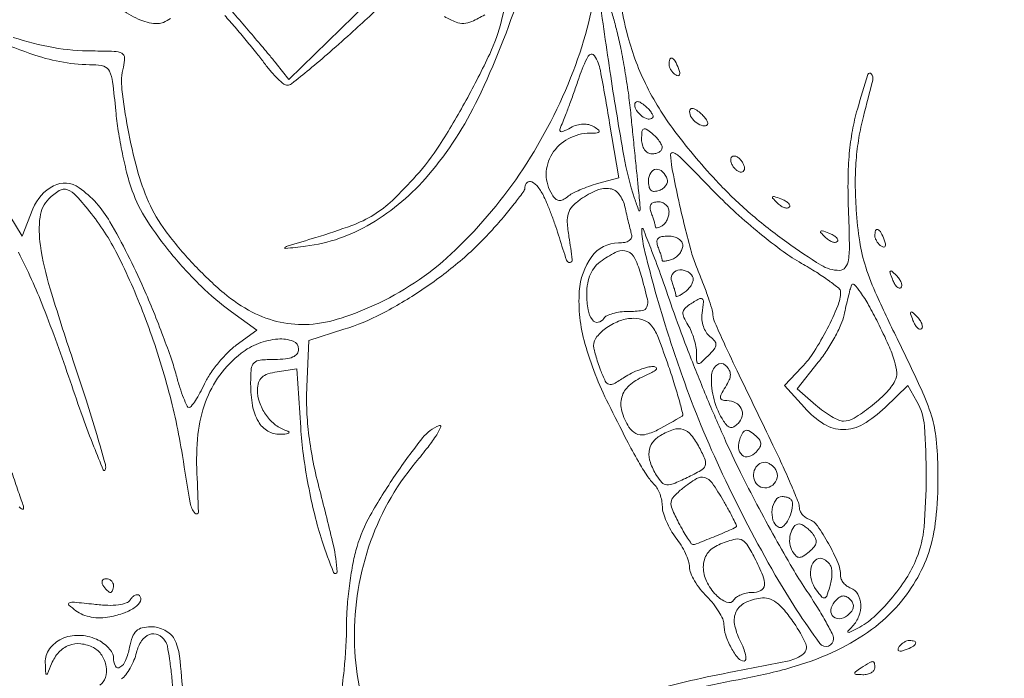
# Model space of a CAD drawing. Units: inches. Extents: x 2656 to 9931, y 1941 to 3068.
# Tile 36 of 46: x 2837 to 2847, y 2967 to 2974. Entities that reach past the tile are written whole.
import ezdxf

# ---------------------------------------------------------------- set-up
doc = ezdxf.new("R2010")
doc.units = ezdxf.units.IN
doc.layers.add('A-ANNO-DIMS', color=2, linetype='Continuous', lineweight=18)
doc.layers.add('A-ELEV-ORN', color=8, linetype='Continuous', lineweight=13)
doc.styles.get("Standard").update_dxf_attribs({"font": 'arial.ttf'})
doc.dimstyles.new('ISO-25', dxfattribs={"dimtxt": 6, "dimasz": 2.5, "dimexe": 1.25, "dimexo": 0.625, "dimtad": 1, "dimdec": 0, "dimlunit": 3, "dimtxsty": 'Standard', "dimcen": 2.5, "dimadec": 0, "dimazin": 0, "dimtfac": 1, "dimtdec": 0, "dimtmove": 0, "dimatfit": 3, "dimfxl": 1, "dimarcsym": 0})

# ---------------------------------------------------------------- blocks, each defined once
blk = doc.blocks.new('*D152')
at = {"layer": 'A-ANNO-DIMS', "color": 0, "lineweight": -2, "transparency": 16777216}
for p, q in [((2847.28, 2990.828), (2707.323, 2990.828)), ((2708.573, 2988.328), (2708.573, 2952.971)), ((2847.248, 2950.471), (2707.323, 2950.471))]:
    blk.add_line(p, q, dxfattribs=at)
at = {"layer": 'A-ANNO-DIMS', "color": 0, "transparency": 16777216}
for points in [[(2708.156, 2988.328), (2708.989, 2988.328), (2708.573, 2990.828)], [(2708.156, 2952.971), (2708.989, 2952.971), (2708.573, 2950.471)]]:
    blk.add_solid(points, dxfattribs=at)
at = {"layer": 'Defpoints', "color": 0, "transparency": 16777216}
for p in [(2847.905, 2990.828), (2708.573, 2950.471), (2847.873, 2950.471)]:
    blk.add_point(p, dxfattribs=at)
at = {"layer": 'A-ANNO-DIMS', "color": 0, "transparency": 16777216, "insert": (2704.843, 2970.649), "char_height": 6, "attachment_point": 5, "rotation": 90}
blk.add_mtext('3\'-4 1/2"', dxfattribs=at)
blk = doc.blocks.new('*D153')
at = {"layer": 'A-ANNO-DIMS', "color": 0, "lineweight": -2, "transparency": 16777216}
for p, q in [((2826.64, 2993.722), (2826.64, 2703.709)), ((2829.546, 2956.424), (2829.546, 2703.709)), ((2824.14, 2704.959), (2821.64, 2704.959)), ((2826.64, 2704.959), (2829.546, 2704.959)), ((2832.046, 2704.959), (2851.745, 2704.959))]:
    blk.add_line(p, q, dxfattribs=at)
at = {"layer": 'A-ANNO-DIMS', "color": 0, "transparency": 16777216}
for points in [[(2824.14, 2705.376), (2824.14, 2704.543), (2826.64, 2704.959)], [(2832.046, 2705.376), (2832.046, 2704.543), (2829.546, 2704.959)]]:
    blk.add_solid(points, dxfattribs=at)
at = {"layer": 'Defpoints', "color": 0, "transparency": 16777216}
for p in [(2826.64, 2994.347), (2829.546, 2957.049), (2829.546, 2704.959)]:
    blk.add_point(p, dxfattribs=at)
at = {"layer": 'A-ANNO-DIMS', "color": 0, "transparency": 16777216, "insert": (2843.145, 2708.65), "char_height": 6, "attachment_point": 5}
blk.add_mtext('0\'-3"', dxfattribs=at)
blk = doc.blocks.new('*D154')
at = {"layer": 'A-ANNO-DIMS', "color": 0, "lineweight": -2, "transparency": 16777216}
for p, q in [((2708.573, 2996.847), (2708.573, 2999.347)), ((2826.015, 2994.347), (2707.323, 2994.347)), ((2708.573, 2994.347), (2708.573, 2990.828)), ((2847.28, 2990.828), (2707.323, 2990.828)), ((2708.573, 2988.328), (2708.573, 2954.647))]:
    blk.add_line(p, q, dxfattribs=at)
at = {"layer": 'A-ANNO-DIMS', "color": 0, "transparency": 16777216}
for points in [[(2708.156, 2996.847), (2708.989, 2996.847), (2708.573, 2994.347)], [(2708.156, 2988.328), (2708.989, 2988.328), (2708.573, 2990.828)]]:
    blk.add_solid(points, dxfattribs=at)
at = {"layer": 'Defpoints', "color": 0, "transparency": 16777216}
for p in [(2826.64, 2994.347), (2708.573, 2990.828), (2847.905, 2990.828)]:
    blk.add_point(p, dxfattribs=at)
at = {"layer": 'A-ANNO-DIMS', "color": 0, "transparency": 16777216, "insert": (2704.843, 2970.237), "char_height": 6, "attachment_point": 5, "rotation": 90}
blk.add_mtext('0\'-3 1/2"', dxfattribs=at)

msp = doc.modelspace()

# ---------------------------------------------------------------- linework, layer by layer
at = {"layer": 'A-ELEV-ORN'}
for points in [[(2842.853, 2974.397, -0.062714), (2842.597, 2973.361, -0.053881), (2842.084, 2972.363, -0.0556), (2841.391, 2971.531, -0.080212), (2840.605, 2970.986, -0.032224), (2840.218, 2970.831, -0.061455), (2839.891, 2970.767, -0.072265), (2839.594, 2970.789, -0.065114), (2839.305, 2970.893, -0.056633), (2839.017, 2971.087, -0.028415), (2838.699, 2971.389, -0.028415), (2838.418, 2971.725, -0.056908), (2838.244, 2972.024, -0.036526), (2838.126, 2972.358, -0.020375), (2838.03, 2972.778, -0.018439), (2837.97, 2973.178, -0.089515), (2837.985, 2973.406, 0.061039), (2837.997, 2973.502, 0.280443), (2837.969, 2973.548, 0.112433), (2837.892, 2973.568, 0.00783), (2837.667, 2973.572, -0.044024), (2837.268, 2973.607, -0.036465), (2836.854, 2973.712, -0.031934)], [(2843.31, 2966.892, -0.021083), (2844.354, 2967.133, 0.026141), (2844.873, 2967.258, 0.039837), (2845.306, 2967.425, 0.045741), (2845.658, 2967.636, 0.058065), (2845.936, 2967.893, 0.04841), (2846.13, 2968.171, 0.05757), (2846.255, 2968.465, 0.049384), (2846.321, 2968.816, 0.024614), (2846.338, 2969.268, 0.021923), (2846.32, 2969.588, 0.049336), (2846.272, 2969.827, 0.034106), (2846.168, 2970.099, 0.006116), (2845.934, 2970.591, -0.007097), (2845.711, 2971.062, -0.029397), (2845.597, 2971.355, -0.039713), (2845.536, 2971.615, -0.021446), (2845.5, 2971.941, -0.015651), (2845.49, 2972.208, -0.020354), (2845.499, 2972.452, -0.021729), (2845.527, 2972.681, -0.023377), (2845.574, 2972.901, 0.004012), (2845.669, 2973.272, 0.238331), (2845.654, 2973.338, 0.595051), (2845.619, 2973.331, 0.00437), (2845.512, 2972.975, 0.026292), (2845.461, 2972.757, 0.0221), (2845.429, 2972.521, 0.019508), (2845.416, 2972.256, 0.012547), (2845.42, 2971.948, -0.005025), (2845.43, 2971.592, -0.041002), (2845.42, 2971.43, -0.122762), (2845.388, 2971.351, -0.238712), (2845.328, 2971.321, -0.138821), (2845.139, 2971.375, -0.018176), (2844.788, 2971.609, -0.021642), (2844.414, 2971.904, -0.026108), (2844.091, 2972.213, -0.027001), (2843.64, 2972.747, -0.048186), (2843.339, 2973.237, -0.051403), (2843.15, 2973.753, -0.035809), (2843.041, 2974.363, 0.011612)], [(2839.024, 2973.936, -0.00618), (2839.13, 2973.816, -0.004408), (2839.245, 2973.68, -0.004451), (2839.353, 2973.547, -0.00948), (2839.433, 2973.443, 0.018291), (2839.501, 2973.358, 0.024307), (2839.569, 2973.286, 0.022933), (2839.63, 2973.233, 0.169618), (2839.666, 2973.22, 0.170059), (2839.71, 2973.236, 0.003586), (2839.892, 2973.383, 0.007897), (2840.104, 2973.563, 0.005188), (2840.342, 2973.776, -0.00338), (2840.721, 2974.118, -0.04635)], [(2841.908, 2974.067), (2841.863, 2973.884, -0.047953), (2841.741, 2973.541, -0.016187), (2841.5, 2973.067, -0.016433), (2841.226, 2972.605, -0.041092), (2840.988, 2972.293, -0.017871), (2840.743, 2972.039, -0.053766), (2840.552, 2971.891, -0.050229), (2840.328, 2971.782, -0.014129), (2839.958, 2971.658, 0.000751), (2839.673, 2971.571, 0.101126), (2839.641, 2971.554, 0.742785), (2839.645, 2971.545, 0.00203), (2839.853, 2971.569, 0.104505), (2840.525, 2971.801, 0.082382), (2841.114, 2972.3, 0.064174), (2841.622, 2973.085, 0.033435), (2842.054, 2974.17, 0.022106)], [(2840.483, 2974.058), (2839.681, 2973.279), (2839.552, 2973.443, 0.007333), (2839.48, 2973.532, 0.001692), (2839.355, 2973.68, 0.001747), (2839.211, 2973.849, 0.001706), (2839.065, 2974.018)], [(2837.973, 2973.995, 0.057004), (2838.163, 2973.889, 0.09937), (2838.34, 2973.853, 0.108281), (2838.395, 2973.865, 0.034437), (2838.468, 2973.905, 0.032541)], [(2841.278, 2973.925, 0.028926), (2841.396, 2973.869, 0.107992), (2841.476, 2973.855, 0.097967), (2841.559, 2973.875, 0.02151), (2841.69, 2973.942)], [(2836.272, 2973.858, 0.029582), (2837.076, 2973.53, 0.082237), (2837.675, 2973.431, -0.074513), (2837.785, 2973.415, -0.207271), (2837.843, 2973.365, -0.084093), (2837.875, 2973.256, -0.006773), (2837.907, 2972.957, 0.015972), (2837.933, 2972.751, 0.011369), (2837.975, 2972.521, 0.011495), (2838.025, 2972.303, 0.023883), (2838.076, 2972.137, 0.057669), (2838.224, 2971.837, 0.028184), (2838.475, 2971.493, 0.027587), (2838.78, 2971.161, 0.036635), (2839.093, 2970.897), (2839.353, 2970.709), (2839.142, 2970.553, 0.038605), (2839.053, 2970.476, 0.023263), (2838.96, 2970.372, 0.023225), (2838.876, 2970.26, 0.037249), (2838.817, 2970.156, -0.013462), (2838.769, 2970.063, -0.020038), (2838.723, 2969.985, -0.015751), (2838.681, 2969.925, -0.236477), (2838.659, 2969.914, -0.294197), (2838.638, 2969.928, -0.012177), (2838.602, 2970.012, -0.017773), (2838.564, 2970.118, -0.011292), (2838.527, 2970.245, 0.018154), (2838.477, 2970.41, 0.00638), (2838.393, 2970.644, 0.006324), (2838.293, 2970.898, 0.007367), (2838.192, 2971.137, 0.027175), (2837.847, 2971.82, 0.106386), (2837.531, 2972.169, 0.282935), (2837.269, 2972.188, 0.181331), (2837.058, 2971.953), (2836.947, 2971.671), (2836.821, 2971.88, 0.042011)], [(2836.908, 2971.506, -0.025971), (2837.163, 2970.944, -0.011782), (2837.439, 2970.186, 0.004309), (2837.569, 2969.813, 0.007894), (2837.683, 2969.511, 0.00415), (2837.779, 2969.273, 0.694448), (2837.799, 2969.274, 0.150521), (2837.8, 2969.33, 0.00245), (2837.712, 2969.637, 0.006144), (2837.602, 2969.994, 0.00401), (2837.467, 2970.404, -0.008425), (2837.234, 2971.133, -0.036079), (2837.134, 2971.577, -0.066195), (2837.13, 2971.868, -0.168907), (2837.22, 2972.055, -0.059645), (2837.328, 2972.139, -0.224773), (2837.411, 2972.148, -0.127121), (2837.501, 2972.087, -0.015227), (2837.657, 2971.901, -0.052466), (2837.939, 2971.454, -0.024343), (2838.213, 2970.822, -0.023509), (2838.441, 2970.114, -0.027309), (2838.59, 2969.422, 0.003756), (2838.671, 2968.934, 0.128056), (2838.719, 2968.828, 0.715598), (2838.754, 2968.84, 0.006631), (2838.739, 2969.238, -0.038668), (2838.75, 2969.638, -0.062097), (2838.827, 2969.971, -0.070148), (2838.974, 2970.245, -0.068088), (2839.192, 2970.47, -0.075108), (2839.37, 2970.571, -0.074118), (2839.57, 2970.616, -0.104512), (2839.725, 2970.595, -0.316192), (2839.782, 2970.512, -0.164293), (2839.767, 2970.465, -0.129352), (2839.724, 2970.432, -0.075863), (2839.649, 2970.413, -0.025511), (2839.536, 2970.407, 0.021968), (2839.386, 2970.4, 0.178574), (2839.325, 2970.371, 0.174885), (2839.296, 2970.309, 0.020892), (2839.29, 2970.156, 0.043336), (2839.309, 2969.933, 0.088805), (2839.369, 2969.77, 0.125073), (2839.466, 2969.671, 0.14633), (2839.591, 2969.639, 0.01274), (2839.658, 2969.643, 0.157257), (2839.681, 2969.652, 0.524361), (2839.679, 2969.665, 0.039035), (2839.642, 2969.682, -0.088287), (2839.533, 2969.744, -0.069673), (2839.442, 2969.844, -0.068701), (2839.381, 2969.967, -0.080851), (2839.36, 2970.096, -0.073644), (2839.372, 2970.171, -0.135274), (2839.404, 2970.223, -0.109805), (2839.465, 2970.258, -0.038951), (2839.562, 2970.28), (2839.764, 2970.309), (2839.803, 2969.707, 0.017712), (2839.831, 2969.426, 0.013084), (2839.881, 2969.116, 0.013118), (2839.947, 2968.811, 0.018296), (2840.023, 2968.543, 0.018649), (2840.141, 2968.221, 0.84301), (2840.176, 2968.229, 0.046019), (2840.138, 2968.499, 0.006058), (2839.999, 2969.062, -0.014444), (2839.932, 2969.352, -0.018534), (2839.888, 2969.623, -0.019852), (2839.866, 2969.879, -0.022359), (2839.866, 2970.126), (2839.888, 2970.602), (2840.247, 2970.716, 0.042983), (2840.632, 2970.875, 0.028302), (2841.045, 2971.12, 0.027738), (2841.439, 2971.417, 0.034228), (2841.769, 2971.738, 0.007807), (2841.897, 2971.885, 0.011327), (2842.005, 2972.019, 0.007101), (2842.091, 2972.134, 0.158019), (2842.103, 2972.173, -0.212493), (2842.126, 2972.222, -0.306704), (2842.172, 2972.229, -0.116091), (2842.237, 2972.175, -0.049272), (2842.298, 2972.077, -0.017168), (2842.333, 2971.998, -0.006886), (2842.376, 2971.888, -0.006804), (2842.419, 2971.768, -0.008541), (2842.456, 2971.655, 0.006236), (2842.529, 2971.425, 0.346324), (2842.565, 2971.402, 0.428109), (2842.588, 2971.43, 0.006685), (2842.554, 2971.664, -0.02305), (2842.537, 2971.815, -0.092243), (2842.548, 2971.907, -0.116837), (2842.589, 2971.978, -0.048286), (2842.674, 2972.05, -0.051712), (2842.842, 2972.144, -0.145026), (2842.975, 2972.159, -0.194836), (2843.07, 2972.1, -0.103782), (2843.128, 2971.972, 0.003398), (2843.146, 2971.891, 0.003194), (2843.166, 2971.809, 0.003177), (2843.184, 2971.737, 0.011017), (2843.197, 2971.69, -0.172957), (2843.196, 2971.655, -0.153568), (2843.172, 2971.627, -0.098751), (2843.126, 2971.608, -0.045369), (2843.062, 2971.602, 0.240793), (2842.787, 2971.462, 0.141871), (2842.66, 2971.107, 0.085228), (2842.718, 2970.57, 0.046137), (2842.959, 2969.95, 0.002777), (2843.145, 2969.581, 0.011089), (2843.266, 2969.359, 0.01768), (2843.356, 2969.213, 0.049192), (2843.432, 2969.121, -0.072159), (2843.462, 2969.08, -0.03806), (2843.488, 2969.023, -0.0369), (2843.505, 2968.959, -0.046713), (2843.512, 2968.898, 0.069701), (2843.522, 2968.83, 0.030218), (2843.553, 2968.745, 0.029173), (2843.598, 2968.656, 0.03429), (2843.651, 2968.578, -0.03034), (2843.704, 2968.501, -0.027752), (2843.748, 2968.417, -0.028834), (2843.78, 2968.337, -0.076098), (2843.79, 2968.276, 0.096524), (2843.803, 2968.215, 0.033427), (2843.843, 2968.135, 0.031738), (2843.9, 2968.05, 0.031897), (2843.967, 2967.974, -0.027616), (2844.035, 2967.899, -0.029667), (2844.092, 2967.818, -0.03103), (2844.132, 2967.744, -0.108485), (2844.143, 2967.691, 0.080423), (2844.162, 2967.577, 0.045303), (2844.218, 2967.448, 0.044022), (2844.289, 2967.342, 0.226965), (2844.351, 2967.312, 0.397473), (2844.368, 2967.327, 0.065356), (2844.364, 2967.375, 0.04263), (2844.344, 2967.444, 0.022195), (2844.307, 2967.526, -0.070131), (2844.252, 2967.691, -0.159908), (2844.269, 2967.82, -0.166772), (2844.359, 2967.91, -0.077793), (2844.518, 2967.959, -0.108309), (2844.6, 2967.954, -0.089808), (2844.679, 2967.914, -0.06072), (2844.763, 2967.834, -0.021767), (2844.862, 2967.702, -0.042697), (2844.983, 2967.488, -0.342151), (2844.958, 2967.385, -0.119272), (2844.812, 2967.316, -0.005091), (2844.248, 2967.204, 0.020325), (2843.366, 2967.002, 0.031031)], [(2840.565, 2966.551, -0.095957), (2840.355, 2967.471, -0.087707), (2840.5, 2968.48, -0.09438), (2840.982, 2969.35, 0.009507), (2841.109, 2969.508, 0.021327), (2841.198, 2969.635, 0.038848), (2841.241, 2969.714, 0.666896), (2841.226, 2969.729, 0.135525), (2841.052, 2969.601, 0.01693), (2840.773, 2969.22, 0.020826), (2840.516, 2968.806, 0.056534), (2840.381, 2968.489, 0.024973), (2840.34, 2968.321, 0.013411), (2840.306, 2968.111, 0.013323), (2840.282, 2967.893, 0.020314), (2840.274, 2967.704, -0.026531), (2840.248, 2967.219, -0.015759), (2840.169, 2966.645, -0.015384)], [(2836.916, 2968.895, 0.046443), (2836.947, 2968.87, 0.495533), (2836.959, 2968.875, 0.152674), (2836.959, 2968.901, 0.013093), (2836.938, 2968.965, -0.007722), (2836.907, 2969.052, -0.000935), (2836.843, 2969.243, -0.001111)], [(2838.598, 2966.947, 0.010925), (2838.56, 2967.362, 0.092946), (2838.506, 2967.541, 0.095655), (2838.468, 2967.588, 0.058053), (2838.409, 2967.628, 0.05525), (2838.338, 2967.655, 0.063506), (2838.266, 2967.664, 0.059093), (2838.177, 2967.653, 0.13444), (2838.118, 2967.621, 0.114543), (2838.078, 2967.559, 0.036658), (2838.049, 2967.453, -0.046905), (2838.008, 2967.318, -0.157361), (2837.95, 2967.248, -0.448318), (2837.903, 2967.261, -0.11211), (2837.883, 2967.349, 0.1326), (2837.871, 2967.395, 0.056806), (2837.832, 2967.448, 0.050694), (2837.775, 2967.497, 0.046624), (2837.708, 2967.536, 0.103136), (2837.528, 2967.576, 0.112073), (2837.353, 2967.54, 0.129566), (2837.228, 2967.437, 0.164796), (2837.184, 2967.296, 0.0025), (2837.188, 2967.185, 0.353585), (2837.196, 2967.176, 0.351009), (2837.207, 2967.182, 0.002485), (2837.249, 2967.285, -0.088994), (2837.323, 2967.402, -0.116417), (2837.427, 2967.473, -0.119244), (2837.55, 2967.489, -0.096506), (2837.677, 2967.45, -0.125381), (2837.763, 2967.372, -0.103427), (2837.808, 2967.256, -0.114975), (2837.801, 2967.142, -0.183925), (2837.743, 2967.066, 0.107671)], [(2837.964, 2967.128, 0.071928), (2838.009, 2967.171, 0.032471), (2838.054, 2967.24, 0.031305), (2838.093, 2967.32, 0.037148), (2838.119, 2967.4, -0.084654), (2838.171, 2967.519, -0.155138), (2838.253, 2967.585, -0.204368), (2838.341, 2967.582, -0.14709), (2838.415, 2967.516, -0.091318), (2838.436, 2967.464, -0.009542), (2838.458, 2967.334, -0.01158), (2838.478, 2967.178, -0.009031), (2838.493, 2967.006, 0.010541)]]:
    msp.add_lwpolyline(points, format="xyb", dxfattribs=at)
for points in [[(2843.046, 2973.776, -0.013205), (2843.086, 2973.598, -0.006854), (2843.127, 2973.373, -0.00681), (2843.163, 2973.142, -0.010294), (2843.187, 2972.939, 0.000202), (2843.207, 2972.741, 0.000153), (2843.229, 2972.523, 0.000154), (2843.25, 2972.318, 0.000358), (2843.265, 2972.165, -0.001534), (2843.285, 2971.967, -0.110402), (2843.281, 2971.935, -0.7056), (2843.27, 2971.935, -0.004671), (2843.227, 2972.06, -0.036376), (2843.117, 2972.496, -0.006701), (2842.982, 2973.315, -0.002798), (2842.858, 2974.173, -0.711672), (2842.906, 2974.198, -0.114458), (2842.927, 2974.165, -0.007415), (2842.965, 2974.057, -0.010497), (2843.006, 2973.924, -0.007618)], [(2842.971, 2972.833), (2843.064, 2972.271), (2842.848, 2972.212, 0.01944), (2842.758, 2972.183, 0.017473), (2842.667, 2972.147, 0.017805), (2842.588, 2972.109, 0.051355), (2842.538, 2972.075, -0.055462), (2842.49, 2972.044, -0.15622), (2842.451, 2972.038, -0.158077), (2842.416, 2972.055, -0.057176), (2842.381, 2972.099, -0.143378), (2842.321, 2972.306, -0.137922), (2842.381, 2972.516, -0.130656), (2842.546, 2972.671, -0.123085), (2842.77, 2972.729, 0.012592), (2842.844, 2972.731, 0.243204), (2842.863, 2972.743, 0.387784), (2842.86, 2972.76, 0.021395), (2842.811, 2972.794, 0.083301), (2842.759, 2972.816, 0.067688), (2842.699, 2972.822, 0.062021), (2842.635, 2972.811, 0.051282), (2842.571, 2972.785, -0.012015), (2842.492, 2972.745, -0.272927), (2842.468, 2972.747, -0.336052), (2842.461, 2972.768, -0.015615), (2842.491, 2972.843, 0.012129), (2842.52, 2972.914, 0.003033), (2842.564, 2973.033, 0.003097), (2842.613, 2973.169, 0.003111), (2842.66, 2973.305, -0.037921), (2842.751, 2973.519, -0.573274), (2842.816, 2973.522, -0.100097), (2842.876, 2973.372, -0.00472)], [(2843.58, 2973.435, 0.088797), (2843.586, 2973.407, 0.053277), (2843.601, 2973.376, 0.051183), (2843.623, 2973.347, 0.061454), (2843.65, 2973.326, 0.1144), (2843.674, 2973.318, 0.32948), (2843.688, 2973.327, 0.155351), (2843.69, 2973.352, 0.036408), (2843.678, 2973.392, 0.029964), (2843.643, 2973.468, 0.168622), (2843.612, 2973.497, 0.444011), (2843.589, 2973.487, 0.079093)], [(2843.411, 2972.887, -0.264952), (2843.365, 2972.874, -0.097357), (2843.302, 2972.904, -0.084765), (2843.248, 2972.961, -0.149534), (2843.229, 2973.022, -0.176123), (2843.237, 2973.045, -0.256649), (2843.257, 2973.053, -0.110288), (2843.291, 2973.041, -0.030483), (2843.336, 2973.008, -0.030935), (2843.375, 2972.971, -0.05004), (2843.402, 2972.935, -0.066988), (2843.416, 2972.905, -0.274667)], [(2843.791, 2972.952, 0.149534), (2843.81, 2972.89, 0.084765), (2843.864, 2972.834, 0.097357), (2843.928, 2972.804, 0.264952), (2843.974, 2972.816, 0.274667), (2843.978, 2972.835, 0.066988), (2843.965, 2972.865, 0.05004), (2843.937, 2972.901, 0.030935), (2843.899, 2972.937, 0.030483), (2843.853, 2972.971, 0.110288), (2843.82, 2972.983, 0.256649), (2843.8, 2972.975, 0.176123)], [(2843.51, 2972.579, -0.167044), (2843.502, 2972.555, -0.095133), (2843.479, 2972.535, -0.075975), (2843.445, 2972.521, -0.056567), (2843.405, 2972.517, -0.132926), (2843.363, 2972.528, -0.107148), (2843.329, 2972.559, -0.089651), (2843.307, 2972.607, -0.064485), (2843.299, 2972.666, -0.02153), (2843.303, 2972.745, -0.243483), (2843.319, 2972.771, -0.285199), (2843.347, 2972.77, -0.027702), (2843.405, 2972.728, -0.031583), (2843.445, 2972.69, -0.034151), (2843.479, 2972.648, -0.036411), (2843.503, 2972.608, -0.117955)], [(2844.939, 2971.393, -0.011671), (2845.092, 2971.301, -0.017384), (2845.221, 2971.214, -0.012556), (2845.322, 2971.137, -0.226393), (2845.339, 2971.101, -0.097548), (2845.31, 2970.956, -0.021009), (2845.203, 2970.722, -0.022913), (2845.069, 2970.489, -0.049851), (2844.942, 2970.326), (2844.764, 2970.141), (2844.968, 2969.913, 0.070733), (2845.168, 2969.744, 0.140656), (2845.366, 2969.688, 0.133051), (2845.571, 2969.743, 0.060285), (2845.795, 2969.913), (2846.029, 2970.14), (2846.123, 2969.975, -0.112118), (2846.2, 2969.722, -0.018342), (2846.217, 2969.207, -0.020283), (2846.195, 2968.686, -0.074855), (2846.119, 2968.367, -0.046499), (2846.012, 2968.159, -0.032722), (2845.855, 2967.947, -0.033275), (2845.68, 2967.764, -0.065122), (2845.515, 2967.649, -0.004388), (2845.435, 2967.609, -0.209201), (2845.418, 2967.608, -0.523579), (2845.415, 2967.618, -0.008587), (2845.462, 2967.669, 0.099511), (2845.527, 2967.773, 0.10171), (2845.546, 2967.894, 0.118463), (2845.516, 2967.998, 0.173667), (2845.444, 2968.06, -0.066404), (2845.404, 2968.082, -0.062204), (2845.37, 2968.114, -0.066541), (2845.347, 2968.152, -0.106625), (2845.339, 2968.188, 0.100816), (2845.312, 2968.322, 0.027214), (2845.216, 2968.517, 0.02503), (2845.102, 2968.699, 0.149487), (2845.015, 2968.767, -0.066359), (2844.977, 2968.787, -0.062579), (2844.946, 2968.817, -0.067076), (2844.924, 2968.851, -0.107584), (2844.917, 2968.884, 0.097311), (2844.907, 2968.938, 0.004626), (2844.838, 2969.107, 0.007446), (2844.75, 2969.306, 0.005277), (2844.646, 2969.528, -0.000529), (2844.299, 2970.247, -0.004156), (2844.141, 2970.583, -0.005965), (2844.051, 2970.785, -0.077965), (2844.031, 2970.864, 0.046602), (2844.018, 2970.931, 0.01196), (2843.984, 2971.037, 0.009849), (2843.934, 2971.176, 0.004445), (2843.862, 2971.356, -0.029497), (2843.81, 2971.508, -0.00682), (2843.742, 2971.768, -0.007038), (2843.672, 2972.071, -0.006934), (2843.61, 2972.376, -0.04477), (2843.597, 2972.508, -0.580404), (2843.631, 2972.528, -0.06677), (2843.719, 2972.459, -0.001932), (2844.051, 2972.12, 0.015764), (2844.267, 2971.912, 0.012488), (2844.513, 2971.699, 0.012678), (2844.752, 2971.514, 0.030532)], [(2844.213, 2972.455, 0.085235), (2844.219, 2972.425, 0.053414), (2844.234, 2972.392, 0.051777), (2844.257, 2972.363, 0.064269), (2844.284, 2972.341, 0.076764), (2844.311, 2972.33, 0.154201), (2844.333, 2972.331, 0.186277), (2844.349, 2972.344, 0.117858), (2844.354, 2972.368, 0.085235), (2844.349, 2972.398, 0.053414), (2844.333, 2972.43, 0.051777), (2844.311, 2972.46, 0.064269), (2844.284, 2972.482, 0.076764), (2844.257, 2972.493, 0.154201), (2844.234, 2972.492, 0.186277), (2844.219, 2972.478, 0.117858)], [(2843.561, 2972.257, -0.142819), (2843.563, 2972.226, -0.094374), (2843.547, 2972.192, -0.080169), (2843.518, 2972.162, -0.065676), (2843.478, 2972.141, -0.081514), (2843.429, 2972.131, -0.202481), (2843.395, 2972.143, -0.158084), (2843.375, 2972.18, -0.046434), (2843.369, 2972.244, -0.135971), (2843.392, 2972.323, -0.244334), (2843.448, 2972.358, -0.216449), (2843.514, 2972.333, -0.117556)], [(2843.58, 2971.923, -0.061875), (2843.575, 2971.881, -0.051278), (2843.56, 2971.839, -0.053305), (2843.537, 2971.802, -0.08825), (2843.51, 2971.778, -0.033138), (2843.483, 2971.764, -0.070413), (2843.46, 2971.757, -0.136025), (2843.446, 2971.759, -0.30111), (2843.44, 2971.768, 0.061959), (2843.437, 2971.788, 0.00979), (2843.427, 2971.825, 0.010735), (2843.413, 2971.868, 0.009199), (2843.397, 2971.913, -0.067159), (2843.386, 2971.961, -0.16701), (2843.394, 2971.996, -0.176865), (2843.421, 2972.017, -0.076855), (2843.467, 2972.024, -0.088448), (2843.511, 2972.017, -0.094811), (2843.547, 2971.995, -0.099989), (2843.572, 2971.962, -0.110744)], [(2844.687, 2972.016, 0.043285), (2844.723, 2971.985, 0.063152), (2844.76, 2971.966, 0.082976), (2844.792, 2971.959, 0.20742), (2844.813, 2971.968, 0.278911), (2844.818, 2971.987, 0.120343), (2844.804, 2972.01, 0.070189), (2844.772, 2972.034, 0.036269), (2844.726, 2972.055, 0.008399), (2844.659, 2972.079, 0.286372), (2844.643, 2972.076, 0.400052), (2844.643, 2972.062, 0.011214)], [(2844.314, 2969.246, 0.006536), (2844.482, 2968.919, 0.005449), (2844.668, 2968.576, 0.005504), (2844.846, 2968.265, 0.014889), (2844.981, 2968.051, -0.008625), (2845.09, 2967.882, -0.011652), (2845.182, 2967.727, -0.008777), (2845.253, 2967.594, -0.113511), (2845.267, 2967.541, -0.733514), (2845.127, 2967.493, -0.027589), (2844.67, 2968.194, -0.020379), (2844.13, 2969.229, -0.025468), (2843.718, 2970.231, -0.007961), (2843.558, 2970.707, -0.009529), (2843.424, 2971.161, -0.008632), (2843.325, 2971.546, -0.056718), (2843.301, 2971.743, -0.824628), (2843.314, 2971.746, -0.005289), (2843.392, 2971.549, -0.00641), (2843.494, 2971.278, -0.003255), (2843.614, 2970.934, 0.009355), (2843.763, 2970.528, 0.005983), (2843.949, 2970.061, 0.006011), (2844.144, 2969.608, 0.011157)], [(2845.179, 2971.664, 0.043285), (2845.216, 2971.633, 0.063152), (2845.252, 2971.614, 0.082976), (2845.284, 2971.608, 0.20742), (2845.306, 2971.616, 0.278911), (2845.31, 2971.635, 0.120343), (2845.296, 2971.658, 0.070189), (2845.264, 2971.682, 0.036269), (2845.219, 2971.703, 0.008399), (2845.151, 2971.728, 0.286372), (2845.136, 2971.724, 0.400052), (2845.135, 2971.71, 0.011214)], [(2845.691, 2971.677, 0.088797), (2845.696, 2971.648, 0.053277), (2845.711, 2971.618, 0.051183), (2845.733, 2971.589, 0.061454), (2845.76, 2971.568, 0.1144), (2845.784, 2971.56, 0.32948), (2845.798, 2971.568, 0.155351), (2845.8, 2971.593, 0.036408), (2845.788, 2971.634, 0.029964), (2845.753, 2971.709, 0.168622), (2845.722, 2971.739, 0.444011), (2845.699, 2971.729, 0.079093)], [(2843.721, 2971.575, -0.096313), (2843.713, 2971.534, -0.06686), (2843.69, 2971.494, -0.064359), (2843.656, 2971.459, -0.074185), (2843.616, 2971.436, -0.02128), (2843.575, 2971.423, -0.039047), (2843.541, 2971.416, -0.053526), (2843.517, 2971.415, -0.388464), (2843.51, 2971.423, 0.066993), (2843.508, 2971.439, 0.007879), (2843.498, 2971.475, 0.009322), (2843.484, 2971.517, 0.007509), (2843.467, 2971.562, -0.076984), (2843.456, 2971.613, -0.207384), (2843.469, 2971.647, -0.16083), (2843.506, 2971.667, -0.043546), (2843.573, 2971.673, -0.064289), (2843.63, 2971.665, -0.082024), (2843.678, 2971.644, -0.098714), (2843.71, 2971.612, -0.149359)], [(2843.295, 2971.268, -0.008166), (2843.358, 2971.026, -0.146921), (2843.354, 2970.947, -0.281036), (2843.306, 2970.908, -0.03242), (2843.163, 2970.899, 0.031897), (2843.08, 2970.894, 0.037484), (2843.004, 2970.878, 0.040811), (2842.942, 2970.855, 0.145171), (2842.912, 2970.828, -0.215467), (2842.852, 2970.788, -0.288446), (2842.794, 2970.812, -0.111054), (2842.75, 2970.917, -0.043385), (2842.736, 2971.075, -0.040311), (2842.746, 2971.189, -0.065478), (2842.774, 2971.283, -0.072227), (2842.822, 2971.359, -0.06225), (2842.893, 2971.423, -0.044955), (2843.05, 2971.513, -0.201976), (2843.153, 2971.516, -0.194483), (2843.231, 2971.444, -0.04145)], [(2843.822, 2971.259, -0.165938), (2843.829, 2971.228, -0.078442), (2843.818, 2971.189, -0.064546), (2843.793, 2971.147, -0.050777), (2843.756, 2971.109, -0.02032), (2843.715, 2971.079, -0.043703), (2843.682, 2971.059, -0.083536), (2843.659, 2971.053, -0.444829), (2843.651, 2971.061, 0.058751), (2843.648, 2971.082, 0.010955), (2843.638, 2971.12, 0.011599), (2843.624, 2971.164, 0.010366), (2843.608, 2971.21, -0.226918), (2843.614, 2971.279, -0.207828), (2843.671, 2971.322, -0.156485), (2843.757, 2971.314, -0.156591)], [(2845.871, 2971.23, 0.036269), (2845.892, 2971.185, 0.070189), (2845.916, 2971.153, 0.120343), (2845.939, 2971.139, 0.278911), (2845.958, 2971.143, 0.20742), (2845.967, 2971.165, 0.082976), (2845.96, 2971.197, 0.063152), (2845.941, 2971.233, 0.043285), (2845.91, 2971.27, 0.011214), (2845.864, 2971.314, 0.400052), (2845.85, 2971.313, 0.286372), (2845.847, 2971.297, 0.008399)], [(2845.897, 2970.187, -0.073578), (2845.804, 2970.062, -0.030404), (2845.645, 2969.921, -0.027996), (2845.478, 2969.805, -0.138904), (2845.368, 2969.774, -0.107398), (2845.321, 2969.784, -0.024624), (2845.247, 2969.822, -0.024357), (2845.165, 2969.876, -0.021635), (2845.085, 2969.939), (2844.893, 2970.104), (2845.111, 2970.378, 0.023663), (2845.198, 2970.499, 0.019915), (2845.279, 2970.634, 0.02038), (2845.343, 2970.764, 0.051134), (2845.375, 2970.864, -0.003739), (2845.395, 2970.952, -0.003523), (2845.416, 2971.041, -0.003503), (2845.436, 2971.12, -0.012214), (2845.451, 2971.17, -0.573587), (2845.478, 2971.176, -0.03485), (2845.543, 2971.097, -0.02498), (2845.627, 2970.964, -0.012213), (2845.721, 2970.787, -0.011133), (2845.832, 2970.554, -0.034203), (2845.893, 2970.39, -0.052561), (2845.915, 2970.271, -0.142539)], [(2843.919, 2970.882, 0.063096), (2843.918, 2970.815, 0.053444), (2843.933, 2970.746, 0.055802), (2843.961, 2970.686, 0.091725), (2843.998, 2970.644, -0.047668), (2844.049, 2970.596, -0.204055), (2844.061, 2970.558, -0.152286), (2844.044, 2970.514, -0.023814), (2843.981, 2970.445, -0.009077), (2843.905, 2970.373, -0.249049), (2843.879, 2970.366, -0.333743), (2843.864, 2970.384, -0.01377), (2843.862, 2970.473, 0.047424), (2843.856, 2970.539, 0.026566), (2843.836, 2970.618, 0.02629), (2843.808, 2970.696, 0.03849), (2843.774, 2970.762, -0.028998), (2843.732, 2970.839, -0.131449), (2843.723, 2970.889, -0.172544), (2843.741, 2970.929, -0.059282), (2843.791, 2970.97, -0.012319), (2843.889, 2971.029, -0.289413), (2843.92, 2971.028, -0.271628), (2843.933, 2970.999, -0.011185)], [(2846.082, 2970.808, 0.036269), (2846.103, 2970.763, 0.070189), (2846.127, 2970.731, 0.120343), (2846.15, 2970.717, 0.278911), (2846.169, 2970.721, 0.20742), (2846.178, 2970.743, 0.082976), (2846.171, 2970.775, 0.063152), (2846.152, 2970.811, 0.043285), (2846.121, 2970.848, 0.011214), (2846.075, 2970.892, 0.400052), (2846.061, 2970.891, 0.286372), (2846.058, 2970.875, 0.008399)], [(2843.576, 2970.336, -0.005887), (2843.638, 2970.146, -0.009599), (2843.686, 2969.983, -0.003722), (2843.722, 2969.844, -0.333408), (2843.715, 2969.826, -0.010559), (2843.463, 2969.684, -0.071779), (2843.329, 2969.635, -0.171214), (2843.241, 2969.647, -0.135889), (2843.169, 2969.712, -0.070909), (2843.096, 2969.877, -0.138718), (2843.096, 2970.02, -0.143801), (2843.171, 2970.139, -0.078468), (2843.317, 2970.232, 0.015267), (2843.404, 2970.273, 0.077614), (2843.448, 2970.304, 0.43872), (2843.447, 2970.323, 0.17295), (2843.42, 2970.334, 0.066995), (2843.36, 2970.327, 0.027137), (2843.28, 2970.302, 0.026258), (2843.197, 2970.267, 0.030223), (2843.122, 2970.224, -0.018027), (2843.013, 2970.157, -0.204318), (2842.964, 2970.152, -0.211036), (2842.927, 2970.184, -0.019328), (2842.878, 2970.298, -0.009763), (2842.851, 2970.375, -0.011128), (2842.828, 2970.449, -0.010358), (2842.811, 2970.512, -0.059653), (2842.807, 2970.547, -0.174874), (2842.841, 2970.641, -0.069459), (2842.944, 2970.735, -0.064373), (2843.081, 2970.805, -0.086156), (2843.218, 2970.829, -0.091788), (2843.328, 2970.808, -0.145187), (2843.404, 2970.75, -0.066639), (2843.472, 2970.625, -0.008413)], [(2844.158, 2970.124, 0.017), (2844.115, 2970.048, 0.15093), (2844.108, 2970.011, 0.309383), (2844.125, 2969.991, 0.065514), (2844.174, 2969.985, -0.119408), (2844.263, 2969.963, -0.160855), (2844.321, 2969.904, -0.173397), (2844.33, 2969.825, -0.139927), (2844.289, 2969.751, -0.058375), (2844.246, 2969.717, -0.179321), (2844.21, 2969.71, -0.163933), (2844.177, 2969.727, -0.047037), (2844.14, 2969.774, -0.077798), (2844.042, 2969.993, -0.075787), (2844.015, 2970.232, -0.200848), (2844.069, 2970.349, -0.401), (2844.161, 2970.346, -0.070398), (2844.198, 2970.298, -0.130049), (2844.209, 2970.251, -0.102822), (2844.197, 2970.196, -0.033857)], [(2843.891, 2969.504, -0.022244), (2843.95, 2969.376, -0.196483), (2843.95, 2969.316, -0.170263), (2843.907, 2969.268, -0.015873), (2843.765, 2969.194, -0.013269), (2843.624, 2969.131, -0.116924), (2843.557, 2969.121, -0.190123), (2843.508, 2969.144, -0.04687), (2843.452, 2969.217, -0.053888), (2843.389, 2969.348, -0.110631), (2843.375, 2969.461, -0.135483), (2843.411, 2969.554, -0.102077), (2843.493, 2969.627, -0.052271), (2843.626, 2969.688, -0.15621), (2843.725, 2969.689, -0.151221), (2843.809, 2969.631, -0.048011)], [(2844.474, 2969.457, -0.139916), (2844.399, 2969.41, -0.255002), (2844.33, 2969.426, -0.202443), (2844.294, 2969.499, -0.104526), (2844.31, 2969.601, -0.044367), (2844.338, 2969.658, -0.203082), (2844.367, 2969.679, -0.192429), (2844.403, 2969.673, -0.039498), (2844.458, 2969.635, -0.045358), (2844.504, 2969.588, -0.151869), (2844.521, 2969.549, -0.158526), (2844.512, 2969.508, -0.050713)], [(2844.674, 2969.275, -0.190717), (2844.689, 2969.192, -0.171854), (2844.644, 2969.118, -0.175934), (2844.563, 2969.089, -0.197141), (2844.487, 2969.121, -0.144911), (2844.45, 2969.188, -0.134859), (2844.455, 2969.267, -0.143758), (2844.498, 2969.328, -0.169916), (2844.565, 2969.352, -0.100929), (2844.592, 2969.346, -0.052079), (2844.623, 2969.329, -0.048757), (2844.652, 2969.305, -0.053016)], [(2844.139, 2968.956, -0.007516), (2844.195, 2968.857, -0.01248), (2844.239, 2968.772, -0.006104), (2844.273, 2968.701, -0.38395), (2844.269, 2968.689, -0.03294), (2844.201, 2968.654, -0.003453), (2844.035, 2968.585, -0.001614), (2843.859, 2968.514, -0.09556), (2843.825, 2968.508, -0.243493), (2843.809, 2968.516, -0.009576), (2843.77, 2968.574, -0.015089), (2843.726, 2968.646, -0.009878), (2843.679, 2968.732, -0.015539), (2843.611, 2968.874, -0.133685), (2843.601, 2968.943, -0.167102), (2843.628, 2969, -0.027846), (2843.72, 2969.084, -0.032379), (2843.862, 2969.184, -0.215032), (2843.946, 2969.195, -0.168413), (2844.021, 2969.14, -0.018582)], [(2844.847, 2968.935, -0.066143), (2844.833, 2968.837, -0.068883), (2844.795, 2968.746, -0.094459), (2844.745, 2968.69, -0.31163), (2844.698, 2968.688, -0.188684), (2844.646, 2968.759, -0.102047), (2844.638, 2968.868, -0.112959), (2844.674, 2968.964, -0.251442), (2844.741, 2969, -0.05931), (2844.781, 2968.995, -0.078243), (2844.816, 2968.981, -0.096657), (2844.838, 2968.96, -0.16037)], [(2845.05, 2968.623, -0.062865), (2845.083, 2968.571, -0.153431), (2845.089, 2968.527, -0.134604), (2845.068, 2968.484, -0.043902), (2845.018, 2968.434, -0.028187), (2844.956, 2968.388, -0.148838), (2844.916, 2968.376, -0.198076), (2844.883, 2968.39, -0.056068), (2844.848, 2968.436, -0.111591), (2844.819, 2968.519, -0.086475), (2844.825, 2968.616, -0.102739), (2844.861, 2968.691, -0.235537), (2844.916, 2968.719, -0.120628), (2844.942, 2968.712, -0.035581), (2844.977, 2968.69, -0.033455), (2845.015, 2968.659, -0.03047)], [(2844.458, 2968.371, -0.019681), (2844.542, 2968.19, -0.12073), (2844.558, 2968.09, -0.269746), (2844.52, 2968.036, -0.109139), (2844.429, 2968.015, 0.049765), (2844.373, 2968.01, 0.04754), (2844.319, 2967.993, 0.051232), (2844.273, 2967.969, 0.106288), (2844.246, 2967.94, -0.36775), (2844.171, 2967.916, -0.106595), (2844.062, 2967.991, -0.075008), (2843.965, 2968.131, -0.114034), (2843.932, 2968.275, -0.068923), (2843.943, 2968.35, -0.081621), (2843.973, 2968.415, -0.080902), (2844.023, 2968.467, -0.066268), (2844.09, 2968.506, -0.021061), (2844.244, 2968.56, -0.163947), (2844.319, 2968.558, -0.165346), (2844.377, 2968.511, -0.021514)], [(2845.234, 2968.296, -0.10575), (2845.247, 2968.258, -0.038364), (2845.25, 2968.201, -0.035955), (2845.244, 2968.136, -0.035598), (2845.229, 2968.072, -0.013446), (2845.197, 2967.979, -0.259301), (2845.174, 2967.96, -0.275389), (2845.147, 2967.969, -0.014837), (2845.089, 2968.044, -0.094127), (2845.041, 2968.144, -0.097115), (2845.034, 2968.253, -0.128566), (2845.068, 2968.335, -0.23627), (2845.131, 2968.367, -0.099466), (2845.157, 2968.362, -0.052279), (2845.186, 2968.346, -0.049076), (2845.213, 2968.323, -0.05395)], [(2837.778, 2968.086, 0.029505), (2837.797, 2968.059, 0.035638), (2837.818, 2968.036, 0.038439), (2837.838, 2968.02, 0.151918), (2837.852, 2968.015, 0.210953), (2837.864, 2968.021, 0.081139), (2837.874, 2968.036, 0.061769), (2837.881, 2968.059, 0.042167), (2837.883, 2968.086, 0.105053), (2837.878, 2968.113, 0.099167), (2837.862, 2968.135, 0.09642), (2837.837, 2968.151, 0.093332), (2837.809, 2968.156, 0.108972), (2837.784, 2968.151, 0.182303), (2837.769, 2968.135, 0.161196), (2837.767, 2968.113, 0.082592)], [(2838.057, 2967.942, -0.171675), (2838.015, 2967.908, -0.053351), (2837.936, 2967.889, -0.039908), (2837.825, 2967.884, -0.019164), (2837.682, 2967.895, 0.00382), (2837.482, 2967.916, 0.111394), (2837.431, 2967.91, 0.562539), (2837.427, 2967.887, 0.026884), (2837.498, 2967.828, 0.063873), (2837.57, 2967.788, 0.051447), (2837.656, 2967.763, 0.048556), (2837.749, 2967.756, 0.04403), (2837.846, 2967.766, 0.038115), (2837.995, 2967.807, 0.069204), (2838.107, 2967.866, 0.125993), (2838.159, 2967.928, 0.318368), (2838.149, 2967.984, 0.181028), (2838.13, 2967.993, 0.12481), (2838.105, 2967.988, 0.090732), (2838.08, 2967.97, 0.056976)], [(2845.429, 2967.796, -0.134871), (2845.345, 2967.748, -0.235304), (2845.268, 2967.765, -0.257458), (2845.24, 2967.834, -0.146109), (2845.276, 2967.919, -0.049888), (2845.319, 2967.961, -0.125124), (2845.358, 2967.979, -0.153701), (2845.396, 2967.974, -0.089272), (2845.434, 2967.948, -0.071603), (2845.463, 2967.91, -0.133832), (2845.471, 2967.874, -0.127288), (2845.46, 2967.836, -0.061647)], [(2845.937, 2967.454, 0.1144), (2845.929, 2967.43, 0.32948), (2845.938, 2967.416, 0.155351), (2845.963, 2967.414, 0.036408), (2846.003, 2967.426, 0.029964), (2846.079, 2967.46, 0.168622), (2846.108, 2967.492, 0.444011), (2846.098, 2967.515, 0.079093), (2846.046, 2967.523, 0.088797), (2846.018, 2967.518, 0.053277), (2845.987, 2967.503, 0.051183), (2845.959, 2967.48, 0.061454)], [(2845.55, 2967.242, 0.011213), (2845.491, 2967.202, 0.309569), (2845.485, 2967.186, 0.327416), (2845.499, 2967.175, 0.011938), (2845.567, 2967.172, 0.055234), (2845.615, 2967.177, 0.075283), (2845.654, 2967.192, 0.095191), (2845.681, 2967.215, 0.17131), (2845.691, 2967.242, 0.042895), (2845.686, 2967.292, 0.364836), (2845.67, 2967.306, 0.137048), (2845.639, 2967.297, 0.007234)]]:
    msp.add_lwpolyline(points, format="xyb", close=True, dxfattribs=at)

# ---------------------------------------------------------------- dimensions: what is measured, and where the dimension line sits
at = {"layer": 'A-ANNO-DIMS'}
for base, p1, p2, picture, middle in [((2708.573, 2990.828), (2826.64, 2994.347), (2847.905, 2990.828), '*D154', (2704.843, 2970.237)), ((2708.573, 2950.471), (2847.905, 2990.828), (2847.873, 2950.471), '*D152', (2704.843, 2970.649))]:
    dim = msp.add_linear_dim(base=base, p1=p1, p2=p2, angle=90, dimstyle='ISO-25', override={"dimdec": 1, "dimlfac": 1, "dimrnd": 0, "dimzin": 1, "dimdsep": 46, "dimlunit": 4, "dimfrac": 2}, dxfattribs=at)
    dim.commit()
    dim.dimension.update_dxf_attribs({"geometry": picture, "text_midpoint": middle})
dim = msp.add_linear_dim(base=(2829.546, 2704.959), p1=(2826.64, 2994.347), p2=(2829.546, 2957.049), dimstyle='ISO-25', override={"dimdec": 1, "dimlfac": 1, "dimrnd": 0, "dimzin": 1, "dimdsep": 46, "dimlunit": 4, "dimfrac": 2}, dxfattribs=at)
dim.commit()
dim.dimension.update_dxf_attribs({"geometry": '*D153', "text_midpoint": (2843.145, 2708.65)})

doc.saveas('drawing.dxf')
